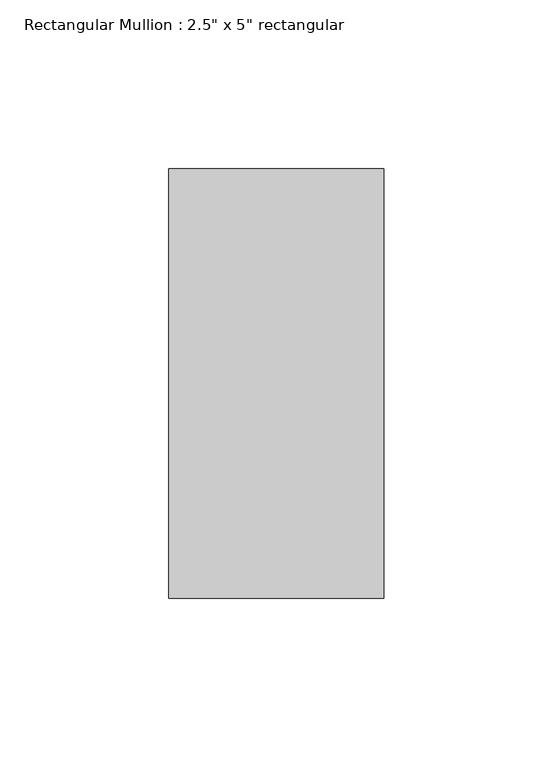
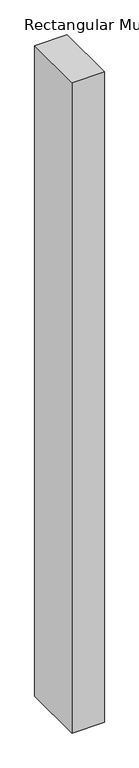
"""IFC4 building model written with IfcOpenShell, lengths in millimetres: member geometry."""

from ifc_helpers import new_model, si_unit, frame, origin, place, context, project, spatial, polyline, outline, extrude, source, transform, mapped, element, save


def member_b14cf619(model_context):
    return source(origin(), model_context, "Body", "SweptSolid", [
        extrude(outline(polyline([(0.0, 63.5), (0.0, -63.5), (-63.5, -63.5), (-63.5, 63.5), (0.0, 63.5)])), frame((0.0, 0.0, -1351.681705), z_axis=(0.0, 0.0, 1.0), x_axis=(1.0, 0.0, 0.0)), (0.0, 0.0, 1.0), 1351.681705),
    ])


if __name__ == "__main__":
    model = new_model("IFC4")
    model_context = context("Model", 3, world=origin())
    ifc_project = project(units=[si_unit("LENGTHUNIT", "METRE", prefix="MILLI")], contexts=[model_context])
    site = spatial("IfcSite", under=ifc_project)
    building = spatial("IfcBuilding", under=site)
    placement = place(None, origin())
    member_shape = member_b14cf619(model_context)
    element("IfcMember", 1, ObjectType="Rectangular Mullion : 2.5\" x 5\" rectangular", at=placement, inside=building, context=model_context, shape_type="MappedRepresentation", body=[
        mapped(member_shape, transform((0.0, 0.0, 0.0), x_axis=(1.0, 0.0, 0.0), y_axis=(0.0, 1.0, 0.0), z_axis=(0.0, 0.0, 1.0))),
    ])
    save(model, "model.ifc")

# Revit data of these elements
# Type "Rectangular Mullion : 2.5\" x 5\" rectangular"
#   built-in parameter 1007304 = 0.416667 (stored number, unit not read)
#   built-in parameter 1007301 = 0.104167 (stored number, unit not read)
#   built-in parameter 1007300 = 0.104167 (stored number, unit not read)
# Element 1 (IfcMember, "Rectangular Mullion : 2.5\" x 5\" rectangular")
#   Materials on its faces: "Iron, Ductile"
# Materials
#   "Iron, Ductile": class "Metal", colour RGB 0 0 0, transparency 0, Description = "Ductile cast iron", Cost = 0
